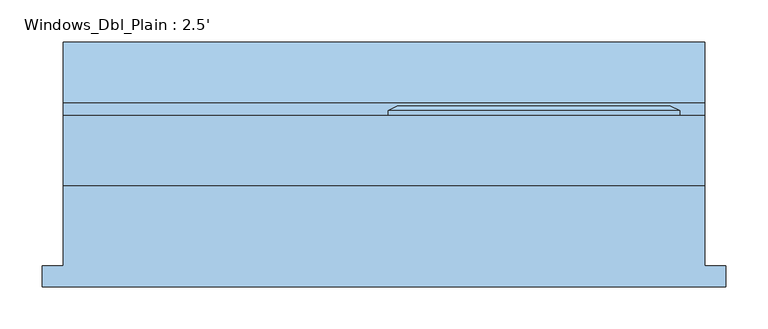
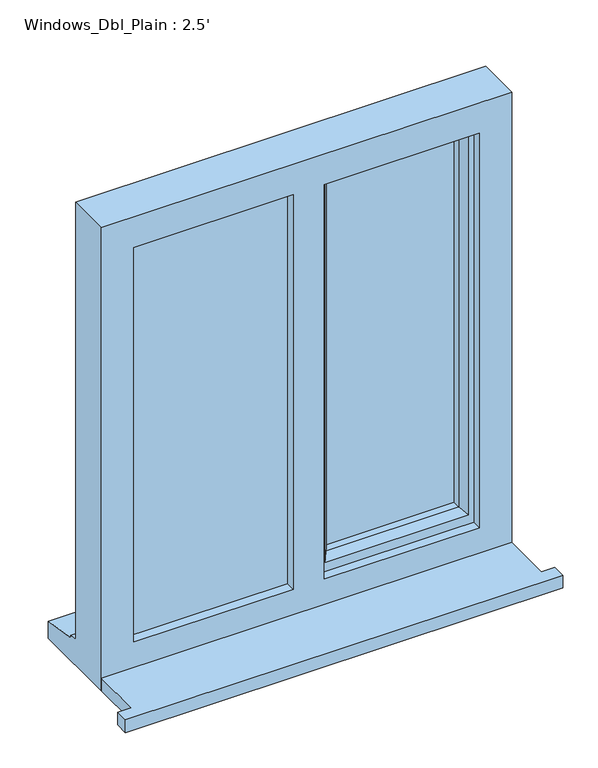
"""IFC4 building model written with IfcOpenShell, lengths in millimetres: window geometry, Windows_Dbl_Plain : 2.5'."""

from ifc_helpers import new_model, si_unit, frame, origin, place, context, project, spatial, polyline, outline, extrude, faceted_brep, source, transform, mapped, element, save


def windows_dbl_plain_2_5_5b7baf13(model_context):
    return source(origin(), model_context, "Body", "SolidModel", [
        extrude(outline(polyline([(-691.0, -130.8434322), (-691.0, -105.8434322), (-666.0, -105.8434322), (-666.0, -10.2434322), (96.0, -10.2434322), (96.0, -105.8434322), (121.0, -105.8434322), (121.0, -130.8434322), (-691.0, -130.8434322)])), frame((0.0, 0.0, 1200.0), z_axis=(0.0, 0.0, 1.0), x_axis=(1.0, 0.0, 0.0)), (0.0, 0.0, 1.0), 25.0),
        faceted_brep([(-280.0, 72.7565678, 2080.0), (-280.0, 78.5300705, 2080.0), (-280.0, 78.5300705, 1253.0), (-280.0, 72.7565678, 1253.0), (-270.0, 7.7565678, 2070.0), (-270.0, 72.7565678, 2070.0), (-270.0, 72.7565678, 1263.0), (-270.0, 7.7565678, 1263.0), (-230.0, 22.2494677, 2030.0), (-240.1480377, 7.7565678, 2040.1480377), (-240.1480377, 7.7565678, 1292.8519623), (-230.0, 22.2494677, 1303.0), (-230.0, 36.7565678, 2030.0), (-230.0, 36.7565678, 1303.0), (-240.0, 60.7565678, 2040.0), (-240.0, 36.7565678, 2040.0), (-240.0, 36.7565678, 1293.0), (-240.0, 60.7565678, 1293.0), (-230.0, 78.5300705, 2030.0), (-230.0, 60.7565678, 2030.0), (-230.0, 60.7565678, 1303.0), (-230.0, 78.5300705, 1303.0), (-247.4457548, 84.3035732, 2047.4457548), (-247.4457548, 84.3035732, 1285.5542452), (-269.2153903, 84.3035732, 2069.2153903), (-269.2153903, 84.3035732, 1263.7846097), (66.0, 78.5300705, 1253.0), (66.0, 72.7565678, 1253.0), (56.0, 72.7565678, 1263.0), (56.0, 7.7565678, 1263.0), (26.1480377, 7.7565678, 1292.8519623), (16.0, 22.2494677, 1303.0), (16.0, 36.7565678, 1303.0), (26.0, 36.7565678, 1293.0), (26.0, 60.7565678, 1293.0), (16.0, 60.7565678, 1303.0), (16.0, 78.5300705, 1303.0), (33.4457548, 84.3035732, 1285.5542452), (55.2153903, 84.3035732, 1263.7846097), (66.0, 78.5300705, 2080.0), (66.0, 72.7565678, 2080.0), (56.0, 72.7565678, 2070.0), (56.0, 7.7565678, 2070.0), (26.1480377, 7.7565678, 2040.1480377), (16.0, 22.2494677, 2030.0), (16.0, 36.7565678, 2030.0), (26.0, 36.7565678, 2040.0), (26.0, 60.7565678, 2040.0), (16.0, 60.7565678, 2030.0), (16.0, 78.5300705, 2030.0), (33.4457548, 84.3035732, 2047.4457548), (55.2153903, 84.3035732, 2069.2153903)], [[[0, 1, 2, 3]], [[4, 5, 6, 7]], [[8, 9, 10, 11]], [[12, 8, 11, 13]], [[14, 15, 16, 17]], [[18, 19, 20, 21]], [[22, 18, 21, 23]], [[1, 24, 25, 2]], [[3, 2, 26, 27]], [[7, 6, 28, 29]], [[11, 10, 30, 31]], [[13, 11, 31, 32]], [[17, 16, 33, 34]], [[21, 20, 35, 36]], [[23, 21, 36, 37]], [[2, 25, 38, 26]], [[27, 26, 39, 40]], [[29, 28, 41, 42]], [[31, 30, 43, 44]], [[32, 31, 44, 45]], [[34, 33, 46, 47]], [[36, 35, 48, 49]], [[37, 36, 49, 50]], [[26, 38, 51, 39]], [[40, 39, 1, 0]], [[3, 27, 40, 0], [5, 41, 28, 6]], [[42, 41, 5, 4]], [[7, 29, 42, 4], [9, 43, 30, 10]], [[44, 43, 9, 8]], [[45, 44, 8, 12]], [[15, 46, 33, 16], [13, 32, 45, 12]], [[47, 46, 15, 14]], [[17, 34, 47, 14], [19, 48, 35, 20]], [[49, 48, 19, 18]], [[50, 49, 18, 22]], [[24, 51, 38, 25], [23, 37, 50, 22]], [[39, 51, 24, 1]]]),
        extrude(outline(polyline([(2050.0, -310.0), (2070.0, -310.0), (2070.0, -626.0), (1263.0, -626.0), (1263.0, -310.0), (1283.0, -310.0), (1283.0, -606.0), (2050.0, -606.0), (2050.0, -310.0)])), frame((0.0, 31.7565678, 0.0), z_axis=(0.0, 1.0, 0.0), x_axis=(0.0, 0.0, 1.0)), (0.0, 0.0, 1.0), 41.0),
        faceted_brep([(96.0, -10.2434322, 2110.0), (-666.0, -10.2434322, 2110.0), (-666.0, -10.2434322, 1200.0), (96.0, -10.2434322, 1200.0), (36.0, -10.2434322, 2050.0), (36.0, -10.2434322, 1275.0), (-252.0, -10.2434322, 1275.0), (-252.0, -10.2434322, 2050.0), (-310.0, -10.2434322, 2050.0), (-310.0, -10.2434322, 1275.0), (-606.0, -10.2434322, 1275.0), (-606.0, -10.2434322, 2050.0), (-666.0, 72.7565678, 2110.0), (-666.0, 72.7565678, 1251.0), (-666.0, 87.7565678, 1249.68767), (-666.0, 87.7565678, 1244.7449676), (-666.0, 160.2565678, 1233.8088847), (-666.0, 160.2565678, 1200.0), (96.0, 72.7565678, 2110.0), (96.0, 72.7565678, 1251.0), (-626.0, 72.7565678, 2070.0), (-626.0, 72.7565678, 1263.0), (-310.0, 72.7565678, 1263.0), (-310.0, 72.7565678, 2070.0), (-270.0, 72.7565678, 2070.0), (-270.0, 72.7565678, 1263.0), (56.0, 72.7565678, 1263.0), (56.0, 72.7565678, 2070.0), (-626.0, 7.7565678, 2070.0), (-626.0, 7.7565678, 1263.0), (-300.0, 7.7565678, 2070.0), (-300.0, 7.7565678, 1263.0), (-310.0, 7.7565678, 2050.0), (-606.0, 7.7565678, 2050.0), (-606.0, 7.7565678, 1275.0), (-310.0, 7.7565678, 1275.0), (-270.0, 7.7565678, 2070.0), (56.0, 7.7565678, 2070.0), (56.0, 7.7565678, 1263.0), (-270.0, 7.7565678, 1263.0), (36.0, 7.7565678, 2050.0), (-252.0, 7.7565678, 2050.0), (-252.0, 7.7565678, 1275.0), (36.0, 7.7565678, 1275.0), (-310.0, 31.7565678, 2070.0), (-300.0, 31.7565678, 2070.0), (96.0, 160.2565678, 1200.0), (96.0, 160.2565678, 1233.8088847), (96.0, 87.7565678, 1244.7449676), (96.0, 87.7565678, 1249.68767), (-300.0, 31.7565678, 1263.0), (-310.0, 31.7565678, 1263.0)], [[[0, 1, 2, 3], [4, 5, 6, 7], [8, 9, 10, 11]], [[2, 1, 12, 13, 14, 15, 16, 17]], [[13, 12, 18, 19], [20, 21, 22, 23], [24, 25, 26, 27]], [[21, 20, 28, 29]], [[28, 30, 31, 29], [32, 33, 34, 35]], [[36, 37, 38, 39], [40, 41, 42, 43]], [[33, 11, 10, 34]], [[1, 0, 18, 12]], [[28, 20, 23, 44, 45, 30]], [[27, 37, 36, 24]], [[11, 33, 32, 8]], [[40, 4, 7, 41]], [[19, 18, 0, 3, 46, 47, 48, 49]], [[27, 26, 38, 37]], [[4, 40, 43, 5]], [[45, 50, 31, 30]], [[50, 45, 44, 51]], [[51, 44, 23, 22]], [[25, 24, 36, 39]], [[41, 7, 6, 42]], [[8, 32, 35, 9]], [[46, 3, 2, 17]], [[47, 46, 17, 16]], [[48, 47, 16, 15]], [[49, 48, 15, 14]], [[19, 49, 14, 13]], [[22, 21, 29, 31, 50, 51]], [[26, 25, 39, 38]], [[6, 5, 43, 42]], [[35, 34, 10, 9]]]),
        extrude(outline(polyline([(-626.0, 31.7565678), (-300.0, 31.7565678), (-300.0, 7.7565678), (-626.0, 7.7565678), (-626.0, 31.7565678)])), frame((0.0, 0.0, 1263.0), z_axis=(0.0, 0.0, 1.0), x_axis=(1.0, 0.0, 0.0)), (0.0, 0.0, 1.0), 807.0),
        extrude(outline(polyline([(26.0, 36.7565678), (-240.0, 36.7565678), (-240.0, 60.7565678), (26.0, 60.7565678), (26.0, 36.7565678)])), frame((0.0, 0.0, 1293.0), z_axis=(0.0, 0.0, 1.0), x_axis=(1.0, 0.0, 0.0)), (0.0, 0.0, 1.0), 747.0),
    ])


if __name__ == "__main__":
    model = new_model("IFC4")
    model_context = context("Model", 3, world=origin())
    ifc_project = project(units=[si_unit("LENGTHUNIT", "METRE", prefix="MILLI")], contexts=[model_context])
    site = spatial("IfcSite", under=ifc_project)
    building = spatial("IfcBuilding", under=site)
    placement = place(None, origin())
    windows_dbl_plain_2_5_shape = windows_dbl_plain_2_5_5b7baf13(model_context)
    element("IfcWindow", 1, ObjectType="Windows_Dbl_Plain : 2.5'", at=placement, inside=building, context=model_context, shape_type="MappedRepresentation", body=[
        mapped(windows_dbl_plain_2_5_shape, transform((0.0, 0.0, 0.0), x_axis=(1.0, 0.0, 0.0), y_axis=(0.0, 1.0, 0.0), z_axis=(0.0, 0.0, 1.0))),
    ])
    save(model, "model.ifc")

# Revit data of these elements
# Type "Windows_Dbl_Plain : 2.5'"
#   Type Mark = "57"
#   Operation = "DoublePanelVertical"
#   Construction Type Id = "GSP4R"
#   Manufacturer = "Revit"
#   Keynote = "L10"
#   Analytic Construction = "1/8 in Pilkington single glazing"
#   Wrap Layers (Ext) from Ext = 0.336286 ft
#   Wrap Layers (Int) from Ext = 0.582349 ft
#   Window Board Projection = 0.082021 ft
#   Window Board Extension = 0.082021 ft
#   Visual Light Transmittance = 0.9
#   Solar Heat Gain Coefficient = 0.78
#   Rough Width = 2.5 ft
#   Rough Height = 2.985564 ft
#   Height = 2.985564 ft
#   Width = 2.5 ft
#   Heat Transfer Coefficient (U) = 3.6886 W/(m²·K)
#   Glazing Thickness = 0.07874 ft
#   FrameOffset - External = 0.164042 ft
#   Frame Depth = 0.213255 ft
#   Default Head Height = 6.922572 ft
#   Cill Depth = 0.287073 ft
#   Cavity Closer Width = 0.164042 ft
#   Cavity Closer Offset from Ext = 0.336286 ft
#   Cavity Closer Depth = 0.278871 ft
#   Vis - Cavity Closers = yes
#   Define Thermal Properties by = 1
#   Material Trim = Window Frame
#   Material Glass = Glass
#   Material Frame = Window Frame
#   Wall Closure = (empty or 0)
# Element 1 (IfcWindow, "Windows_Dbl_Plain : 2.5'")
#   Materials on its faces: "Window Frame", "Glass"
# Materials
#   "Window Frame": colour RGB 249 249 249, transparency 0, Keynote = "L10", Cost = 0
#   "Glass": class "Glass", colour RGB 0 128 192, transparency 0.9, Description = "Soda Lime Glass", Cost = 0
